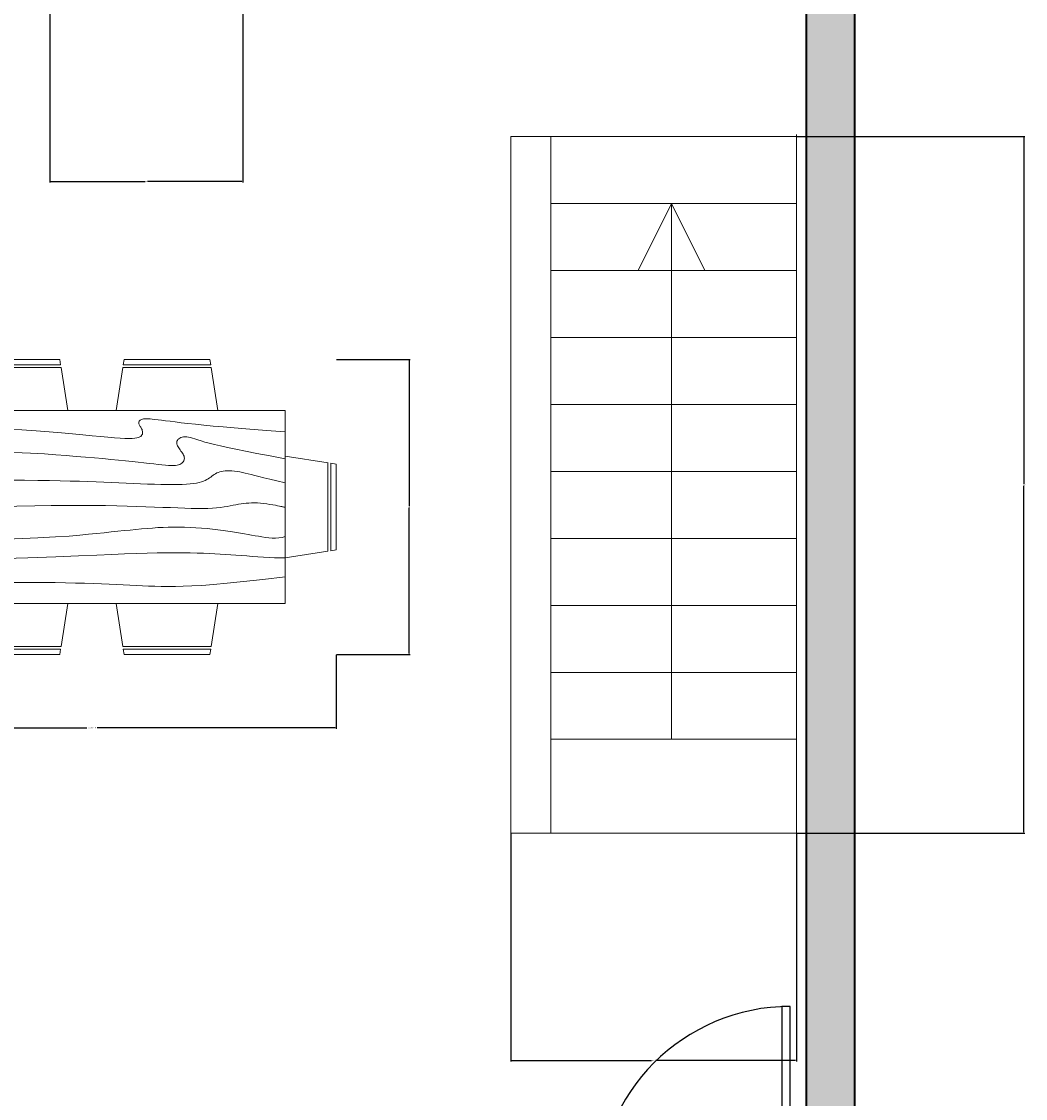
# Model space of a CAD drawing. Units: inches. Extents: x 1563 to 2428, y 777 to 1464.
# Tile 7 of 11: x 1810 to 1997, y 1063 to 1263. Entities that reach past the tile are written whole.
import ezdxf

# ---------------------------------------------------------------- set-up
doc = ezdxf.new("R2010")
doc.units = ezdxf.units.IN
for name, color, linetype, lineweight in [('A-ANNO-DIMS', 2, 'Continuous', 18), ('A-DOOR', 4, 'Continuous', 25), ('A-FLOR-STRS', 7, 'Continuous', 18), ('A-FURN', 9, 'Continuous', 18), ('A-WALL', 7, 'Continuous', 35), ('A-WALL-PATT', 8, 'Continuous', 13)]:
    doc.layers.add(name, color=color, linetype=linetype, lineweight=lineweight)
doc.styles.get("Standard").update_dxf_attribs({"font": 'arial.ttf'})
doc.dimstyles.get("Standard").update_dxf_attribs({"dimtxt": 0.18, "dimasz": 0.18, "dimexe": 0.18, "dimexo": 0.0625, "dimgap": 0.09, "dimtad": 0, "dimtih": 1, "dimtoh": 1, "dimdec": 4, "dimzin": 0, "dimdsep": 46, "dimtxsty": 'Standard', "dimcen": 0.09, "dimadec": 0, "dimazin": 0, "dimtfac": 1, "dimtdec": 4, "dimtofl": 0, "dimtmove": 0, "dimatfit": 3, "dimfxl": 1, "dimtolj": 1, "dimtzin": 0, "dimarcsym": 0})

# ---------------------------------------------------------------- blocks, each defined once
blk = doc.blocks.new('*U3')
for p, q in [((0, 0), (0, -6)), ((-40, 0), (-40, -6))]:
    blk.add_line(p, q)
blk.add_lwpolyline([(0, 0), (0, 40), (-1.75, 40), (-1.75, 0)], close=True)
blk.add_arc((0, 0), 40, 90, 180)
blk = doc.blocks.new('Dining Set - 36 x 72 in.')
for p, q in [((-22, 27.5), (-22.1562, 26.50042)), ((-5.8416, 26.5), (-22.1534, 26.5)), ((-22, 27.5), (-6, 27.5)), ((-5.8437, 26.49966), (-6, 27.5)), ((6, 27.5), (5.8438, 26.50042)), ((22.1584, 26.5), (5.8466, 26.5)), ((6, 27.5), (22, 27.5)), ((22.1563, 26.49966), (22, 27.5)), ((-22.2343, 26.00059), (-23.4847, 17.99762)), ((-22.2304, 26), (-5.7608, 26)), ((-4.5152, 17.99762), (-5.7655, 25.99926)), ((5.7657, 26.00059), (4.5153, 17.99762)), ((5.7696, 26), (22.2392, 26)), ((23.4848, 17.99762), (22.2345, 25.99926)), ((36, 18), (-36, 18)), ((-36, 18), (-36, -18)), ((36, -18), (36, 18)), ((-45.5, 8), (-44.5004, 8.15617)), ((-44.5, -8.15843), (-44.5, 8.15338)), ((-44.0006, 8.23428), (-35.9976, 9.48474)), ((-44, 8.23041), (-44, -8.23915)), ((44.0006, 8.23428), (35.9976, 9.48474)), ((44, 8.23041), (44, -8.23915)), ((44.5, -8.15843), (44.5, 8.15338)), ((45.5, 8), (44.5005, 8.15617)), ((-45.5, 8), (-45.5, -8)), ((45.5, 8), (45.5, -8)), ((-44.4997, -8.15631), (-45.5, -8)), ((44.4997, -8.15631), (45.5, -8)), ((-35.9976, -9.48476), (-43.9993, -8.2345)), ((35.9976, -9.48476), (43.9993, -8.2345)), ((-36, -18), (36, -18)), ((-22.2343, -26.0006), (-23.4847, -17.99762)), ((-4.5152, -17.99762), (-5.7655, -25.99928)), ((5.7657, -26.0006), (4.5153, -17.99762)), ((23.4848, -17.99762), (22.2345, -25.99928)), ((-22.2304, -26), (-5.7608, -26)), ((5.7696, -26), (22.2392, -26)), ((-22, -27.5), (-22.1562, -26.50044)), ((-5.8416, -26.5), (-22.1534, -26.5)), ((-22, -27.5), (-6, -27.5)), ((-5.8437, -26.49967), (-6, -27.5)), ((6, -27.5), (5.8438, -26.50044)), ((22.1584, -26.5), (5.8466, -26.5)), ((6, -27.5), (22, -27.5)), ((22.1563, -26.49967), (22, -27.5))]:
    blk.add_line(p, q)
for points in [[(-36, 15), (-31.1772, 14.97754), (-26.8079, 14.91406), (-22.8538, 14.81543), (-19.276, 14.6875), (-16.0362, 14.53613), (-13.0957, 14.36718), (-10.4159, 14.18652), (-7.9583, 14), (-5.6904, 13.81315), (-3.6035, 13.63021), (-1.6954, 13.45508), (0.0365, 13.29166), (1.5945, 13.14388), (2.9811, 13.01562), (4.1988, 12.9108), (5.25, 12.83333), (6.1393, 12.78613), (6.8802, 12.76823), (7.4883, 12.77767), (7.9792, 12.8125), (8.3685, 12.87077), (8.6719, 12.95052), (8.9049, 13.0498), (9.0833, 13.16666), (9.2205, 13.29899), (9.3216, 13.44401), (9.3895, 13.59879), (9.4271, 13.76041), (9.4373, 13.92594), (9.4232, 14.09245), (9.3875, 14.257), (9.3333, 14.41666), (9.2638, 14.56917), (9.1836, 14.71484), (9.0975, 14.85465), (9.0104, 14.98958), (8.9272, 15.1206), (8.8529, 15.2487), (8.7922, 15.37483), (8.75, 15.5), (8.7305, 15.62467), (8.7344, 15.74739), (8.7617, 15.86621), (8.8125, 15.97916), (8.8867, 16.08431), (8.9844, 16.17968), (9.1055, 16.26334), (9.25, 16.33333), (9.4189, 16.38802), (9.6172, 16.42708), (9.8506, 16.45052), (10.125, 16.45833), (10.4463, 16.45052), (10.8203, 16.42708), (11.2529, 16.38802), (11.75, 16.33333), (12.3184, 16.26318), (12.9694, 16.17838), (13.7151, 16.07991), (14.5677, 15.96875), (15.5395, 15.84586), (16.6426, 15.71224), (17.8893, 15.56884), (19.2917, 15.41666), (20.859, 15.25667), (22.5879, 15.08984), (24.4721, 14.91715), (26.5052, 14.73958), (28.6809, 14.5581), (30.9929, 14.3737), (33.4347, 14.18733), (36, 14)], [(-36, 10), (-28.9766, 10.14274), (-23.1725, 10.20442), (-18.4241, 10.19775), (-14.5677, 10.13541), (-11.4399, 10.03011), (-8.877, 9.89453), (-6.7154, 9.74137), (-4.7917, 9.58333), (-2.9698, 9.43082), (-1.2246, 9.28515), (0.4415, 9.14534), (2.026, 9.01041), (3.5266, 8.87939), (4.9408, 8.7513), (6.266, 8.62516), (7.5, 8.5), (8.6411, 8.37549), (9.6914, 8.2539), (10.6538, 8.13818), (11.5312, 8.03125), (12.3267, 7.93603), (13.043, 7.85547), (13.6831, 7.79248), (14.25, 7.75), (14.7471, 7.7303), (15.1797, 7.73307), (15.5537, 7.75732), (15.875, 7.80208), (16.1494, 7.86637), (16.3828, 7.94922), (16.5811, 8.04964), (16.75, 8.16666), (16.8944, 8.29915), (17.0143, 8.44531), (17.1089, 8.60319), (17.1771, 8.77083), (17.218, 8.94629), (17.2305, 9.1276), (17.2137, 9.31282), (17.1667, 9.5), (17.0895, 9.6875), (16.987, 9.875), (16.8649, 10.0625), (16.7292, 10.25), (16.5856, 10.4375), (16.4401, 10.625), (16.2985, 10.8125), (16.1667, 11), (16.05, 11.18733), (15.9518, 11.3737), (15.8752, 11.5581), (15.8229, 11.73958), (15.798, 11.91715), (15.8034, 12.08984), (15.842, 12.25667), (15.9167, 12.41666), (16.0295, 12.56836), (16.1784, 12.70833), (16.3605, 12.83268), (16.5729, 12.9375), (16.8127, 13.01888), (17.0768, 13.07291), (17.3625, 13.0957), (17.6667, 13.08333), (17.9894, 13.03312), (18.3418, 12.94726), (18.7382, 12.82918), (19.1927, 12.68229), (19.7195, 12.51001), (20.3327, 12.31575), (21.0465, 12.10294), (21.875, 11.875), (22.8357, 11.63354), (23.959, 11.37304), (25.2786, 11.08618), (26.8282, 10.76562), (28.6414, 10.40405), (30.752, 9.99414), (33.1936, 9.52856), (36, 9)], [(-36, 5.5), (-30.7157, 5.3348), (-26.069, 5.20963), (-21.9946, 5.11767), (-18.4271, 5.05208), (-15.3009, 5.00602), (-12.5508, 4.97265), (-10.1112, 4.94515), (-7.9167, 4.91666), (-5.909, 4.88167), (-4.0586, 4.83984), (-2.3429, 4.79215), (-0.7396, 4.73958), (0.7739, 4.6831), (2.22, 4.6237), (3.6213, 4.56233), (5, 4.5), (6.373, 4.43782), (7.7344, 4.3776), (9.0723, 4.32129), (10.375, 4.27083), (11.6309, 4.22819), (12.8281, 4.19531), (13.9551, 4.17415), (15, 4.16666), (15.954, 4.17448), (16.819, 4.19791), (17.6001, 4.23698), (18.3021, 4.29166), (18.9299, 4.36198), (19.4883, 4.44791), (19.9823, 4.54948), (20.4167, 4.66666), (20.7969, 4.79899), (21.1302, 4.94401), (21.4245, 5.09879), (21.6875, 5.26041), (21.9271, 5.42594), (22.1511, 5.59245), (22.3672, 5.757), (22.5834, 5.91666), (22.8065, 6.06868), (23.0404, 6.21093), (23.2879, 6.34147), (23.5521, 6.45833), (23.8358, 6.55957), (24.142, 6.64323), (24.4735, 6.70735), (24.8334, 6.75), (25.2235, 6.76969), (25.642, 6.76692), (26.0858, 6.74267), (26.5521, 6.69791), (27.0379, 6.63362), (27.5404, 6.55078), (28.0565, 6.45036), (28.5834, 6.33333), (29.1242, 6.19987), (29.7071, 6.04687), (30.3661, 5.87044), (31.1354, 5.66666), (32.0493, 5.43164), (33.142, 5.16146), (34.4475, 4.85221), (36, 4.5)], [(-36, -1), (-30.7915, -0.6591), (-26.0195, -0.38216), (-21.6519, -0.16284), (-17.6563, 0.00521), (-14.0005, 0.12833), (-10.6523, 0.21289), (-7.5796, 0.26522), (-4.75, 0.29166), (-2.134, 0.29793), (0.2878, 0.28711), (2.5317, 0.26163), (4.6146, 0.22396), (6.5529, 0.17651), (8.3633, 0.12174), (10.0623, 0.06209), (11.6667, 0), (13.1899, -0.06201), (14.6341, -0.1211), (15.9982, -0.17432), (17.2813, -0.21875), (18.4823, -0.25147), (19.6003, -0.26953), (20.6343, -0.27002), (21.5834, -0.25), (22.4481, -0.20768), (23.2357, -0.14584), (23.9549, -0.06836), (24.6146, 0.02083), (25.2235, 0.11784), (25.7904, 0.21875), (26.3241, 0.31966), (26.8334, 0.41666), (27.3265, 0.50618), (27.8099, 0.58593), (28.2894, 0.65397), (28.7709, 0.70833), (29.2601, 0.74707), (29.763, 0.76823), (30.2855, 0.76985), (30.8334, 0.75), (31.4088, 0.70784), (31.9994, 0.64713), (32.589, 0.57275), (33.1615, 0.48958), (33.7008, 0.4025), (34.1908, 0.3164), (34.6153, 0.23616), (34.9584, 0.16666), (35.2099, 0.11165), (35.3848, 0.07031), (35.504, 0.04069), (35.5886, 0.02083), (35.6594, 0.00879), (35.7377, 0.0026), (35.8442, 0.00032), (36, 0)], [(-36, -6.5), (-27.1843, -6.31267), (-20.084, -6.1263), (-14.469, -5.9419), (-10.1094, -5.76042), (-6.7752, -5.58285), (-4.2363, -5.41016), (-2.2629, -5.24333), (-0.625, -5.08334), (0.8708, -4.93099), (2.2715, -4.78646), (3.5872, -4.64974), (4.8281, -4.52084), (6.0046, -4.39974), (7.127, -4.28646), (8.2053, -4.18099), (9.25, -4.08334), (10.2705, -3.99382), (11.2734, -3.91407), (12.2647, -3.84603), (13.25, -3.79167), (14.2354, -3.75293), (15.2266, -3.73177), (16.2295, -3.73015), (17.25, -3.75), (18.2912, -3.79248), (19.3451, -3.85547), (20.4009, -3.93604), (21.4479, -4.03125), (22.4754, -4.13819), (23.4727, -4.25391), (24.4289, -4.37549), (25.3334, -4.5), (26.1785, -4.62492), (26.9694, -4.74935), (27.7145, -4.87281), (28.4219, -4.99479), (29.1, -5.11483), (29.7572, -5.23242), (30.4016, -5.34709), (31.0417, -5.45834), (31.6837, -5.56437), (32.3262, -5.65821), (32.9658, -5.73153), (33.599, -5.77604), (34.2224, -5.78345), (34.8327, -5.74545), (35.4264, -5.65373), (36, -5.5)], [(-36, -10), (-26.4022, -9.81299), (-18.4675, -9.62891), (-11.9839, -9.45069), (-6.7396, -9.28125), (-2.5226, -9.12354), (0.8789, -8.98047), (3.6769, -8.85498), (6.0833, -8.75), (8.2767, -8.66765), (10.3021, -8.60677), (12.1712, -8.56543), (13.8958, -8.54167), (15.4876, -8.53353), (16.9583, -8.53907), (18.3197, -8.55632), (19.5834, -8.58334), (20.7616, -8.61841), (21.8685, -8.66081), (22.9188, -8.71004), (23.9271, -8.76563), (24.9081, -8.82707), (25.8763, -8.89388), (26.8465, -8.96558), (27.8334, -9.04167), (28.8474, -9.12118), (29.8828, -9.20117), (30.93, -9.27824), (31.9792, -9.34896), (33.0205, -9.40991), (34.0443, -9.45768), (35.0407, -9.48885), (36, -9.5)], [(-36, -14.5), (-30.0881, -14.33513), (-25.0332, -14.21224), (-20.7312, -14.12647), (-17.0781, -14.07292), (-13.97, -14.04671), (-11.3027, -14.04297), (-8.9724, -14.05681), (-6.875, -14.08334), (-4.9224, -14.11833), (-3.0905, -14.16016), (-1.3709, -14.20785), (0.2448, -14.26042), (1.7647, -14.3169), (3.1973, -14.3763), (4.5507, -14.43767), (5.8333, -14.5), (7.0554, -14.5621), (8.235, -14.62175), (9.3922, -14.67652), (10.5469, -14.72396), (11.7192, -14.76164), (12.929, -14.78711), (14.1965, -14.79794), (15.5417, -14.79167), (16.9933, -14.76424), (18.6152, -14.70508), (20.4804, -14.60197), (22.6615, -14.44271), (25.2312, -14.21509), (28.2624, -13.9069), (31.8277, -13.50594), (36, -13)]]:
    blk.add_lwpolyline(points)
blk = doc.blocks.new('*D42')
at = {"layer": 'A-ANNO-DIMS', "color": 0, "lineweight": -2, "transparency": 16777216}
for p, q in [((1777.49, 1145.29), (1777.49, 1131.52)), ((1868.49, 1145.29), (1868.49, 1131.52)), ((1777.67, 1131.7), (1822.03, 1131.7)), ((1868.31, 1131.7), (1823.94, 1131.7))]:
    blk.add_line(p, q, dxfattribs=at)
at = {"layer": 'A-ANNO-DIMS', "color": 0, "transparency": 16777216}
for points in [[(1777.67, 1131.73), (1777.67, 1131.67), (1777.49, 1131.7)], [(1868.31, 1131.73), (1868.31, 1131.67), (1868.49, 1131.7)]]:
    blk.add_solid(points, dxfattribs=at)
at = {"layer": 'Defpoints', "color": 0, "transparency": 16777216}
for p in [(1777.49, 1145.35), (1868.49, 1145.35), (1868.49, 1131.7)]:
    blk.add_point(p, dxfattribs=at)
at = {"layer": 'A-ANNO-DIMS', "color": 0, "transparency": 16777216, "insert": (1822.99, 1131.7), "char_height": 0.18, "attachment_point": 5}
blk.add_mtext('\\A1;DINING SET 91', dxfattribs=at)
blk = doc.blocks.new('*D43')
at = {"layer": 'A-ANNO-DIMS', "color": 0, "lineweight": -2, "transparency": 16777216}
for p, q in [((1868.55, 1200.35), (1882.32, 1200.35)), ((1882.14, 1200.17), (1882.14, 1173.03)), ((1882.14, 1145.53), (1882.14, 1172.67)), ((1868.55, 1145.35), (1882.32, 1145.35))]:
    blk.add_line(p, q, dxfattribs=at)
at = {"layer": 'A-ANNO-DIMS', "color": 0, "transparency": 16777216}
for points in [[(1882.11, 1200.17), (1882.17, 1200.17), (1882.14, 1200.35)], [(1882.11, 1145.53), (1882.17, 1145.53), (1882.14, 1145.35)]]:
    blk.add_solid(points, dxfattribs=at)
at = {"layer": 'Defpoints', "color": 0, "transparency": 16777216}
for p in [(1868.49, 1200.35), (1882.14, 1200.35), (1868.49, 1145.35)]:
    blk.add_point(p, dxfattribs=at)
at = {"layer": 'A-ANNO-DIMS', "color": 0, "transparency": 16777216, "insert": (1882.14, 1172.85), "char_height": 0.18, "attachment_point": 5}
blk.add_mtext('\\A1;55', dxfattribs=at)
blk = doc.blocks.new('*D64')
at = {"layer": 'A-ANNO-DIMS', "color": 0, "lineweight": -2, "transparency": 16777216}
for p, q in [((1815.11, 1275.87), (1815.11, 1233.35)), ((1851.11, 1275.87), (1851.11, 1233.35)), ((1815.29, 1233.53), (1832.89, 1233.53)), ((1850.93, 1233.53), (1833.32, 1233.53))]:
    blk.add_line(p, q, dxfattribs=at)
at = {"layer": 'A-ANNO-DIMS', "color": 0, "transparency": 16777216}
for points in [[(1815.29, 1233.56), (1815.29, 1233.5), (1815.11, 1233.53)], [(1850.93, 1233.56), (1850.93, 1233.5), (1851.11, 1233.53)]]:
    blk.add_solid(points, dxfattribs=at)
at = {"layer": 'Defpoints', "color": 0, "transparency": 16777216}
for p in [(1815.11, 1275.93), (1851.11, 1275.93), (1815.11, 1233.53)]:
    blk.add_point(p, dxfattribs=at)
at = {"layer": 'A-ANNO-DIMS', "color": 0, "transparency": 16777216, "insert": (1833.11, 1233.53), "char_height": 0.18, "attachment_point": 5}
blk.add_mtext('\\A1;36', dxfattribs=at)
blk = doc.blocks.new('*D67')
at = {"layer": 'A-ANNO-DIMS', "color": 0, "lineweight": -2, "transparency": 16777216}
for p, q in [((1901.06, 1112.03), (1901.06, 1069.51)), ((1954.3, 1112.03), (1954.3, 1069.51)), ((1901.24, 1069.69), (1927.28, 1069.69)), ((1954.12, 1069.69), (1928.07, 1069.69))]:
    blk.add_line(p, q, dxfattribs=at)
at = {"layer": 'A-ANNO-DIMS', "color": 0, "transparency": 16777216}
for points in [[(1901.24, 1069.72), (1901.24, 1069.66), (1901.06, 1069.69)], [(1954.12, 1069.72), (1954.12, 1069.66), (1954.3, 1069.69)]]:
    blk.add_solid(points, dxfattribs=at)
at = {"layer": 'Defpoints', "color": 0, "transparency": 16777216}
for p in [(1901.06, 1112.09), (1954.3, 1112.09), (1901.06, 1069.69)]:
    blk.add_point(p, dxfattribs=at)
at = {"layer": 'A-ANNO-DIMS', "color": 0, "transparency": 16777216, "insert": (1927.68, 1069.69), "char_height": 0.18, "attachment_point": 5}
blk.add_mtext('\\A1;53.24', dxfattribs=at)
blk = doc.blocks.new('*D68')
at = {"layer": 'A-ANNO-DIMS', "color": 0, "lineweight": -2, "transparency": 16777216}
for p, q in [((1954.36, 1241.89), (1996.88, 1241.89)), ((1996.7, 1241.71), (1996.7, 1177.17)), ((1996.7, 1112.27), (1996.7, 1176.81)), ((1954.36, 1112.09), (1996.88, 1112.09))]:
    blk.add_line(p, q, dxfattribs=at)
at = {"layer": 'A-ANNO-DIMS', "color": 0, "transparency": 16777216}
for points in [[(1996.67, 1241.71), (1996.73, 1241.71), (1996.7, 1241.89)], [(1996.67, 1112.27), (1996.73, 1112.27), (1996.7, 1112.09)]]:
    blk.add_solid(points, dxfattribs=at)
at = {"layer": 'Defpoints', "color": 0, "transparency": 16777216}
for p in [(1954.3, 1241.89), (1954.3, 1112.09), (1996.7, 1112.09)]:
    blk.add_point(p, dxfattribs=at)
at = {"layer": 'A-ANNO-DIMS', "color": 0, "transparency": 16777216, "insert": (1996.7, 1176.99), "char_height": 0.18, "attachment_point": 5}
blk.add_mtext('\\A1;129.8', dxfattribs=at)

msp = doc.modelspace()

# ---------------------------------------------------------------- hatches: boundary and pattern name
at = {"layer": 'A-WALL-PATT'}
h = msp.add_hatch(color=256, dxfattribs=at)
h.dxf.hatch_style = 1
h.paths.add_polyline_path([(1965.105, 1421.428), (1605.105, 1421.428), (1605.105, 821.428), (1965.105, 821.428)])
h.paths.add_polyline_path([(1614.105, 1199.428), (1704.105, 1199.428), (1738.605, 1199.428), (1738.605, 1251.928), (1734.105, 1251.928), (1734.105, 1203.928), (1704.105, 1203.928), (1614.105, 1203.928), (1614.105, 1335.928), (1665.105, 1335.928), (1665.105, 1340.428), (1614.105, 1340.428), (1614.105, 1412.428), (1704.105, 1412.428), (1704.105, 1340.428), (1701.105, 1340.428), (1701.105, 1335.928), (1704.105, 1335.928), (1768.605, 1335.928), (1768.605, 1340.428), (1708.605, 1340.428), (1708.605, 1412.428), (1807.605, 1412.428), (1807.605, 1340.428), (1804.605, 1340.428), (1804.605, 1335.928), (1807.605, 1335.928), (1807.605, 1275.928), (1815.105, 1275.928), (1815.105, 1280.428), (1812.105, 1280.428), (1812.105, 1412.428), (1956.105, 1412.428), (1956.105, 1280.428), (1854.105, 1280.428), (1854.105, 1275.928), (1956.105, 1275.928), (1956.105, 830.428), (1614.105, 830.428)], flags=16)
h.paths.add_polyline_path([(1917.224, 1038.928), (1917.224, 1043.846, -0.4014527), (1951.591, 1079.751), (1951.591, 1079.786), (1953.163, 1079.786), (1953.163, 1043.846), (1953.163, 1038.455), (1953.105, 1034.428), (1953.105, 1038.928), (1953.163, 1043.846), (1951.591, 1043.846), (1951.591, 1079.751, 0.4014527), (1917.224, 1043.846), (1917.224, 1038.455), (1917.224, 1034.428), (1834.605, 1034.428), (1834.605, 906.928), (1858.605, 906.928), (1858.605, 954.928), (1932.105, 954.928), (1932.105, 902.428), (1834.605, 902.428), (1834.605, 1034.428), (1914.224, 1034.428), (1914.224, 1038.928)], flags=0)
edge = h.paths.add_edge_path(flags=0)
edge.add_ellipse((1674.345, 1004.483), major_axis=(1.48, 0), ratio=0.8423039, start_angle=90, end_angle=180, ccw=False)
edge.add_line((1674.345, 1005.73), (1674.921, 1005.73))
edge.add_ellipse((2202.617, 985.642), major_axis=(528.234, 0), ratio=0.8423039, start_angle=176.34957, end_angle=177.82005, ccw=False)
edge.add_ellipse((1739.278, 760.804), major_axis=(-313.308, 0), ratio=0.8423039, start_angle=-77.87403, end_angle=-76.21947, ccw=False)
edge.add_ellipse((1739.278, 767.659), major_axis=(305.303, 0), ratio=0.8423039, start_angle=100.20954, end_angle=102.44463, ccw=False)
edge.add_ellipse((1659.357, 1231.328), major_axis=(250.96, 0), ratio=0.8423039, start_angle=-80.74343, end_angle=-77.44507)
edge.add_line((1705.625, 1023.567), (1711.685, 1026.918))
edge.add_ellipse((1711.754, 1026.21), major_axis=(0.74, 0), ratio=0.8423039, start_angle=52.06687, end_angle=90, ccw=False)
edge.add_line((1712.16, 1026.731), (1717.882, 1023.567))
edge.add_ellipse((1764.151, 1231.328), major_axis=(250.96, 0), ratio=0.8423039, start_angle=257.44507, end_angle=260.74343)
edge.add_ellipse((1684.229, 767.659), major_axis=(305.303, 0), ratio=0.8423039, start_angle=77.55537, end_angle=79.79046, ccw=False)
edge.add_ellipse((1684.229, 760.804), major_axis=(-313.308, 0), ratio=0.8423039, start_angle=256.21947, end_angle=257.87403, ccw=False)
edge.add_ellipse((1220.891, 985.642), major_axis=(-528.234, 0), ratio=0.8423039, start_angle=182.17995, end_angle=183.65043, ccw=False)
edge.add_line((1748.586, 1005.73), (1749.162, 1005.73))
edge.add_ellipse((1749.162, 1004.483), major_axis=(-1.48, 0), ratio=0.8423039, start_angle=180, end_angle=270, ccw=False)
edge.add_line((1750.642, 1004.483), (1750.642, 980.28))
edge.add_ellipse((1749.162, 980.28), major_axis=(1.48, 0), ratio=0.8423039, start_angle=270, end_angle=360, ccw=False)
edge.add_ellipse((-8843.864, 962.352), major_axis=(10593.026, 0), ratio=0.84230387, start_angle=-0.3241203, end_angle=0.0902291, ccw=False)
edge.add_ellipse((-8843.864, 962.352), major_axis=(10593.026, 0), ratio=0.84230387, start_angle=-0.3838668, end_angle=-0.3241203, ccw=False)
edge.add_ellipse((1749.162, 890.136), major_axis=(1.48, 0), ratio=0.8423039, start_angle=0, end_angle=90, ccw=False)
edge.add_line((1750.642, 890.136), (1750.642, 865.933))
edge.add_ellipse((1749.162, 865.933), major_axis=(1.48, 0), ratio=0.8423039, start_angle=270, end_angle=360, ccw=False)
edge.add_line((1749.162, 864.686), (1748.528, 864.686))
edge.add_ellipse((-8843.864, 962.352), major_axis=(10593.026, 0), ratio=0.84230387, start_angle=-0.6186432, end_angle=-0.5282715, ccw=False)
edge.add_ellipse((1747.592, 846.206), major_axis=(-2.22, 0), ratio=0.8423039, start_angle=179.37176, end_angle=248.46476, ccw=False)
edge.add_ellipse((-8844.604, 962.352), major_axis=(-10595.313, 0), ratio=0.842303864, start_angle=179.3534459, end_angle=179.3717628, ccw=False)
edge.add_ellipse((1744.512, 842.854), major_axis=(-5.246, 0), ratio=0.8423039, start_angle=90, end_angle=179.35345, ccw=False)
edge.add_line((1744.512, 838.435), (1678.995, 838.435))
edge.add_ellipse((1678.995, 842.854), major_axis=(5.246, 0), ratio=0.8423039, start_angle=180.64655, end_angle=270, ccw=False)
edge.add_ellipse((12268.111, 962.352), major_axis=(-10595.313, 0), ratio=0.84230387, start_angle=0.6282372, end_angle=0.6465541, ccw=False)
edge.add_ellipse((1675.916, 846.206), major_axis=(-2.22, 0), ratio=0.8423039, start_angle=-68.46476, end_angle=0.62824, ccw=False)
edge.add_ellipse((12267.371, 962.352), major_axis=(-10593.026, 0), ratio=0.84230387, start_angle=0.5282715, end_angle=0.6465541, ccw=False)
edge.add_line((1674.98, 864.686), (1674.345, 864.686))
edge.add_ellipse((1674.345, 865.933), major_axis=(-1.48, 0), ratio=0.8423039, start_angle=0, end_angle=90, ccw=False)
edge.add_line((1672.865, 865.933), (1672.865, 890.136))
edge.add_ellipse((1674.345, 890.136), major_axis=(1.48, 0), ratio=0.8423039, start_angle=90, end_angle=180, ccw=False)
edge.add_ellipse((12267.371, 962.352), major_axis=(-10593.026, 0), ratio=0.84230387, start_angle=0.3241203, end_angle=0.3838668, ccw=False)
edge.add_ellipse((12267.371, 962.352), major_axis=(-10593.026, 0), ratio=0.84230387, start_angle=-0.0902291, end_angle=0.3241203, ccw=False)
edge.add_ellipse((1674.345, 980.28), major_axis=(-1.48, 0), ratio=0.8423039, start_angle=0, end_angle=90, ccw=False)
edge.add_line((1672.865, 980.28), (1672.865, 1004.483))
h.paths.add_polyline_path([(1622.542, 1135.584), (1648.534, 1136.233), (1648.683, 1130.234), (1647.126, 1130.196), (1648.323, 1082.21), (1649.88, 1082.249), (1650.03, 1076.251), (1624.038, 1075.603, -0.266667)], flags=0)
edge = h.paths.add_edge_path(flags=0)
edge.add_line((1694.584, 990.705), (1700.334, 994.711))
edge.add_line((1700.334, 994.711), (1702.248, 994.711))
edge.add_line((1702.248, 994.711), (1702.248, 997.061))
edge.add_ellipse((1758.417, 997.061), major_axis=(56.169, 0), ratio=0.8423039, start_angle=150.56143, end_angle=180, ccw=False)
edge.add_ellipse((1665.091, 997.061), major_axis=(-56.169, 0), ratio=0.8423039, start_angle=180, end_angle=209.43857, ccw=False)
edge.add_line((1721.26, 997.061), (1721.26, 994.711))
edge.add_line((1721.26, 994.711), (1723.174, 994.711))
edge.add_line((1723.174, 994.711), (1728.923, 990.705))
edge.add_line((1728.923, 990.705), (1728.923, 975.895))
edge.add_ellipse((1725.091, 976.043), major_axis=(0.357, 6.34), ratio=0.6038336, start_angle=106.34259, end_angle=270.99799, ccw=False)
edge.add_line((1721.26, 975.15), (1721.26, 997.061))
edge.add_ellipse((1665.091, 997.061), major_axis=(-56.169, 0), ratio=0.8423039, start_angle=180, end_angle=209.43857)
edge.add_ellipse((1758.417, 997.061), major_axis=(56.169, 0), ratio=0.8423039, start_angle=150.56143, end_angle=180)
edge.add_line((1702.248, 997.061), (1702.248, 975.15))
edge.add_ellipse((1698.416, 976.043), major_axis=(-0.357, 6.34), ratio=0.6038336, start_angle=89.00201, end_angle=253.65741, ccw=False)
edge.add_line((1694.584, 975.895), (1694.584, 990.705))
edge = h.paths.add_edge_path(flags=0)
edge.add_line((1675.832, 952.075), (1679.883, 938.848))
edge.add_ellipse((5378.107, 931.045), major_axis=(-3698.236, 0), ratio=0.84230387, start_angle=-0.120897, end_angle=0.364076)
edge.add_line((1679.976, 907.545), (1676.149, 892.52))
edge.add_ellipse((12267.371, 962.352), major_axis=(10591.546, 0), ratio=0.84230387, start_angle=180.3241656, end_angle=180.3777642, ccw=False)
edge.add_ellipse((12267.371, 962.352), major_axis=(10591.546, 0), ratio=0.84230387, start_angle=180.0555943, end_angle=180.3241656, ccw=False)
edge = h.paths.add_edge_path(flags=0)
edge.add_ellipse((1706.366, 891.542), major_axis=(81.773, 0), ratio=0.8423039, start_angle=94.27742, end_angle=111.83495, ccw=False)
edge.add_line((1701.225, 960.283), (1722.283, 960.283))
edge.add_ellipse((1717.141, 891.542), major_axis=(-81.773, 0), ratio=0.8423039, start_angle=248.16505, end_angle=265.72258, ccw=False)
edge.add_line((1743.29, 956.803), (1741.105, 940.427))
edge.add_ellipse((1714.553, 877.238), major_axis=(79.58, 0), ratio=0.8423039, start_angle=67.20809, end_angle=85.12993)
edge.add_line((1720.25, 944.097), (1703.258, 944.097))
edge.add_ellipse((1708.954, 877.238), major_axis=(79.58, 0), ratio=0.8423039, start_angle=94.87007, end_angle=112.79191)
edge.add_line((1682.403, 940.427), (1680.218, 956.803))
h.paths.add_polyline_path([(1664.992, 1093.991), (1664.992, 1123.991), (1724.992, 1123.991), (1724.992, 1093.991)], flags=0)
h.paths.add_polyline_path([(1716.588, 1099.729), (1715.404, 1099.805), (1715.021, 1099.823), (1716.177, 1099.758)], flags=0)
h.paths.add_polyline_path([(1711.325, 1103.757), (1712.167, 1103.706), (1713.009, 1103.642), (1713.84, 1103.566), (1715.041, 1103.439), (1716.532, 1103.244), (1717.793, 1103.048), (1718.876, 1102.854), (1719.676, 1102.699), (1720.157, 1102.605), (1720.632, 1102.513), (1721.109, 1102.424), (1721.595, 1102.339), (1722.088, 1102.264), (1722.585, 1102.205), (1723.082, 1102.17), (1723.575, 1102.164), (1724.321, 1102.211), (1724.533, 1102.268), (1723.842, 1102.16), (1722.864, 1102.172), (1721.894, 1102.287), (1720.935, 1102.454), (1720.157, 1102.605), (1719.676, 1102.699), (1719.18, 1102.795), (1718.66, 1102.892), (1718.109, 1102.991), (1717.517, 1103.091), (1716.876, 1103.191), (1716.179, 1103.29), (1715.435, 1103.387), (1714.652, 1103.48), (1713.84, 1103.566), (1713.009, 1103.642), (1712.167, 1103.706), (1711.325, 1103.757), (1710.492, 1103.791), (1709.676, 1103.806), (1708.873, 1103.805), (1707.707, 1103.78), (1707.292, 1103.757), (1708.499, 1103.805), (1710.086, 1103.807)], flags=0)
h.paths.add_polyline_path([(1713.959, 1106.591), (1714.651, 1106.624), (1715.279, 1106.674), (1715.852, 1106.736), (1716.373, 1106.807), (1716.851, 1106.885), (1717.289, 1106.966), (1717.696, 1107.046), (1718.341, 1107.178), (1719.173, 1107.331), (1720.169, 1107.421), (1721.131, 1107.383), (1722.032, 1107.286), (1722.934, 1107.152), (1723.887, 1106.983), (1724.746, 1106.795), (1724.72, 1106.798), (1724.663, 1106.807), (1724.241, 1106.906), (1724.159, 1106.924), (1723.885, 1106.979), (1723.546, 1107.044), (1723.157, 1107.113), (1722.732, 1107.182), (1722.284, 1107.249), (1721.827, 1107.308), (1721.375, 1107.357), (1720.942, 1107.391), (1720.539, 1107.406), (1720.162, 1107.405), (1719.804, 1107.388), (1719.459, 1107.357), (1719.12, 1107.314), (1718.781, 1107.259), (1718.435, 1107.195), (1718.076, 1107.124), (1717.402, 1106.986), (1716.59, 1106.837), (1715.56, 1106.696), (1714.317, 1106.598)], flags=0)
h.paths.add_polyline_path([(1708.692, 1110.124), (1709.455, 1110.13), (1710.147, 1110.149), (1710.772, 1110.18), (1711.334, 1110.224), (1711.836, 1110.28), (1712.283, 1110.349), (1712.678, 1110.43), (1713.026, 1110.524), (1713.33, 1110.63), (1713.596, 1110.746), (1713.832, 1110.87), (1714.042, 1110.999), (1714.234, 1111.131), (1714.413, 1111.264), (1714.586, 1111.396), (1715.065, 1111.75), (1715.879, 1112.11), (1716.842, 1112.224), (1717.903, 1112.165), (1719.048, 1111.965), (1719.867, 1111.736), (1720.686, 1111.487), (1721.596, 1111.22), (1721.917, 1111.136), (1721.028, 1111.383), (1720.222, 1111.628), (1719.815, 1111.75), (1719.434, 1111.857), (1719.054, 1111.951), (1718.672, 1112.031), (1718.292, 1112.097), (1717.918, 1112.149), (1717.554, 1112.185), (1717.204, 1112.204), (1716.871, 1112.206), (1716.559, 1112.191), (1716.271, 1112.156), (1716.006, 1112.105), (1715.761, 1112.038), (1715.534, 1111.957), (1715.323, 1111.864), (1715.125, 1111.759), (1714.937, 1111.645), (1714.759, 1111.524), (1714.586, 1111.396), (1714.413, 1111.264), (1714.003, 1110.96), (1713.331, 1110.606), (1712.501, 1110.382), (1711.61, 1110.245), (1710.489, 1110.158), (1709.111, 1110.121)], flags=0)
h.paths.add_polyline_path([(1707.127, 1113.075), (1707.639, 1113.025), (1708.092, 1112.991), (1708.49, 1112.975), (1708.836, 1112.977), (1709.135, 1112.996), (1709.392, 1113.032), (1709.612, 1113.084), (1709.798, 1113.15), (1709.957, 1113.23), (1710.092, 1113.324), (1710.208, 1113.431), (1710.304, 1113.554), (1710.379, 1113.698), (1710.434, 1113.866), (1710.467, 1114.062), (1710.477, 1114.289), (1710.463, 1114.553), (1710.426, 1114.857), (1710.364, 1115.202), (1710.282, 1115.58), (1710.184, 1115.98), (1710.076, 1116.391), (1709.961, 1116.801), (1709.844, 1117.201), (1709.731, 1117.579), (1709.626, 1117.924), (1709.532, 1118.228), (1709.454, 1118.493), (1709.392, 1118.723), (1709.351, 1118.924), (1709.293, 1119.435), (1709.831, 1119.942), (1710.705, 1120.121), (1711.507, 1119.898), (1712.224, 1119.567), (1713.189, 1119.016), (1713.529, 1118.804), (1712.958, 1119.148), (1712.468, 1119.428), (1712.046, 1119.649), (1711.683, 1119.817), (1711.366, 1119.937), (1711.084, 1120.016), (1710.826, 1120.057), (1710.582, 1120.067), (1710.354, 1120.049), (1710.142, 1120.006), (1709.951, 1119.941), (1709.781, 1119.857), (1709.635, 1119.757), (1709.516, 1119.645), (1709.426, 1119.524), (1709.366, 1119.395), (1709.335, 1119.255), (1709.331, 1119.1), (1709.351, 1118.924), (1709.392, 1118.723), (1709.454, 1118.493), (1709.52, 1118.268), (1709.799, 1117.356), (1710.028, 1116.57), (1710.245, 1115.749), (1710.45, 1114.804), (1710.477, 1114.289), (1710.448, 1113.654), (1709.908, 1113.153), (1709.165, 1112.979), (1708.318, 1112.974), (1707.448, 1113.039)], flags=0)
h.paths.add_polyline_path([(1700.892, 1119.857), (1701.604, 1119.819), (1702.196, 1119.805), (1702.683, 1119.813), (1703.076, 1119.841), (1703.387, 1119.887), (1703.63, 1119.951), (1703.816, 1120.03), (1703.959, 1120.124), (1704.069, 1120.23), (1704.15, 1120.346), (1704.204, 1120.47), (1704.234, 1120.599), (1704.242, 1120.731), (1704.231, 1120.864), (1704.202, 1120.996), (1704.159, 1121.124), (1704.103, 1121.246), (1704.039, 1121.362), (1703.97, 1121.474), (1703.901, 1121.582), (1703.834, 1121.687), (1703.775, 1121.79), (1703.564, 1122.226), (1704.048, 1122.698), (1704.756, 1122.769), (1705.49, 1122.723), (1706.24, 1122.641), (1706.547, 1122.601), (1706.092, 1122.657), (1705.695, 1122.701), (1705.348, 1122.732), (1705.049, 1122.751), (1704.792, 1122.757), (1704.573, 1122.751), (1704.386, 1122.732), (1704.227, 1122.701), (1704.092, 1122.657), (1703.977, 1122.601), (1703.88, 1122.534), (1703.802, 1122.458), (1703.742, 1122.374), (1703.702, 1122.284), (1703.68, 1122.188), (1703.677, 1122.09), (1703.692, 1121.991), (1703.726, 1121.89), (1703.769, 1121.802), (1704.039, 1121.362), (1704.301, 1120.887), (1704.133, 1120.165), (1703.43, 1119.866), (1702.481, 1119.798), (1701.306, 1119.827)], flags=0)
edge = h.paths.add_edge_path(flags=0)
edge.add_ellipse((1711.754, 1009.752), major_axis=(-147.018, 0), ratio=0.8423039, start_angle=76.40187, end_angle=103.59813)
edge.add_line((1741.105, 888.411), (1741.105, 869.587))
edge.add_ellipse((1711.754, 990.928), major_axis=(-147.018, 0), ratio=0.8423039, start_angle=76.40187, end_angle=103.59813, ccw=False)
edge.add_line((1682.403, 869.587), (1682.403, 888.411))
edge = h.paths.add_edge_path(flags=0)
edge.add_ellipse((-8843.864, 962.352), major_axis=(-10591.546, 0), ratio=0.84230387, start_angle=179.6758344, end_angle=179.9444057, ccw=False)
edge.add_ellipse((-8843.864, 962.352), major_axis=(-10591.546, 0), ratio=0.84230387, start_angle=179.6222358, end_angle=179.6758344, ccw=False)
edge.add_line((1747.358, 892.52), (1743.531, 907.545))
edge.add_ellipse((-1954.6, 931.045), major_axis=(3698.236, 0), ratio=0.84230387, start_angle=-0.364076, end_angle=0.120897)
edge.add_line((1743.625, 938.848), (1747.676, 952.075))
h.paths.add_polyline_path([(1637.931, 1162.087), (1637.931, 1188.087, -0.1904762), (1721.931, 1188.087), (1721.931, 1162.087), (1715.931, 1162.087), (1715.931, 1163.644), (1643.931, 1163.644), (1643.931, 1162.087)], flags=0)
h.paths.add_polyline_path([(1667.931, 1189.491, -0.0496282), (1691.931, 1189.491), (1691.931, 1182.705), (1667.931, 1182.705)], flags=0)
edge = h.paths.add_edge_path(flags=0)
edge.add_ellipse((1685.362, 859.825), major_axis=(-2.96, 0), ratio=0.8423039, start_angle=-90, end_angle=0, ccw=False)
edge.add_line((1685.362, 862.318), (1738.145, 862.318))
edge.add_ellipse((1738.145, 859.825), major_axis=(2.96, 0), ratio=0.8423039, start_angle=0, end_angle=90, ccw=False)
edge.add_line((1741.105, 859.825), (1741.105, 840.361))
edge.add_line((1741.105, 840.361), (1682.403, 840.361))
edge.add_line((1682.403, 840.361), (1682.403, 859.825))
h.paths.add_polyline_path([(1777.486, 1164.853), (1777.486, 1180.853), (1778.486, 1181.01), (1778.486, 1164.697)], flags=0)
h.paths.add_polyline_path([(1786.986, 1154.853), (1786.986, 1163.369), (1778.986, 1164.619), (1778.986, 1181.088), (1786.986, 1182.338), (1786.986, 1190.853), (1799.502, 1190.853), (1800.752, 1198.853), (1817.221, 1198.853), (1818.471, 1190.853), (1827.502, 1190.853), (1828.752, 1198.853), (1845.221, 1198.853), (1846.471, 1190.853), (1858.986, 1190.853), (1858.986, 1182.338), (1866.986, 1181.088), (1866.986, 1164.619), (1858.986, 1163.369), (1858.986, 1154.853), (1846.471, 1154.853), (1845.221, 1146.853), (1828.752, 1146.853), (1827.502, 1154.853), (1818.471, 1154.853), (1817.221, 1146.853), (1800.752, 1146.853), (1799.502, 1154.853)], flags=0)
h.paths.add_polyline_path([(1800.986, 1145.353), (1800.83, 1146.353), (1817.143, 1146.353), (1816.986, 1145.353)], flags=0)
h.paths.add_polyline_path([(1851.408, 1167.858), (1852.086, 1167.738), (1852.744, 1167.621), (1853.388, 1167.506), (1854.028, 1167.395), (1854.67, 1167.289), (1855.313, 1167.195), (1855.952, 1167.122), (1856.585, 1167.077), (1857.209, 1167.07), (1858.147, 1167.128), (1858.413, 1167.2), (1857.547, 1167.066), (1856.312, 1167.08), (1855.07, 1167.223), (1854.028, 1167.395), (1853.388, 1167.506), (1852.744, 1167.621), (1852.086, 1167.738), (1851.408, 1167.858), (1850.288, 1168.052), (1849.956, 1168.104), (1850.701, 1167.98)], flags=0)
h.paths.add_polyline_path([(1845.435, 1172.646), (1846.222, 1172.707), (1846.941, 1172.785), (1847.601, 1172.874), (1848.21, 1172.971), (1848.777, 1173.072), (1849.311, 1173.173), (1850.14, 1173.331), (1851.063, 1173.483), (1852.014, 1173.591), (1853.012, 1173.633), (1854.075, 1173.594), (1855.251, 1173.473), (1856.4, 1173.306), (1857.391, 1173.132), (1857.945, 1173.02), (1858.196, 1172.965), (1858.595, 1172.871), (1858.575, 1172.874), (1858.49, 1172.894), (1858.371, 1172.924), (1858.196, 1172.965), (1857.945, 1173.02), (1857.602, 1173.089), (1857.177, 1173.17), (1856.687, 1173.256), (1856.148, 1173.343), (1855.575, 1173.426), (1854.986, 1173.5), (1854.395, 1173.561), (1853.82, 1173.603), (1853.272, 1173.623), (1852.749, 1173.622), (1852.247, 1173.6), (1851.757, 1173.562), (1851.276, 1173.507), (1850.796, 1173.439), (1850.313, 1173.359), (1849.82, 1173.27), (1849.311, 1173.173), (1848.421, 1173.005), (1847.25, 1172.818), (1845.826, 1172.665)], flags=0)
h.paths.add_polyline_path([(1840.587, 1177.09), (1841.289, 1177.145), (1841.916, 1177.215), (1842.475, 1177.301), (1842.969, 1177.403), (1843.403, 1177.52), (1843.783, 1177.652), (1844.117, 1177.797), (1844.411, 1177.952), (1844.674, 1178.114), (1844.914, 1178.279), (1845.138, 1178.446), (1845.644, 1178.831), (1846.285, 1179.221), (1847.125, 1179.521), (1847.998, 1179.624), (1848.834, 1179.619), (1849.768, 1179.529), (1850.775, 1179.363), (1851.78, 1179.14), (1852.111, 1179.053), (1851.57, 1179.187), (1851.043, 1179.304), (1850.527, 1179.404), (1850.024, 1179.487), (1849.539, 1179.551), (1849.072, 1179.596), (1848.628, 1179.62), (1848.21, 1179.623), (1847.82, 1179.603), (1847.46, 1179.561), (1847.128, 1179.497), (1846.822, 1179.413), (1846.539, 1179.312), (1846.274, 1179.195), (1846.027, 1179.064), (1845.793, 1178.922), (1845.57, 1178.77), (1845.354, 1178.61), (1844.817, 1178.201), (1844.106, 1177.764), (1843.208, 1177.452), (1842.225, 1177.25), (1840.973, 1177.11)], flags=0)
h.paths.add_polyline_path([(1836.67, 1180.646), (1837.236, 1180.603), (1837.734, 1180.584), (1838.166, 1180.586), (1838.54, 1180.611), (1838.861, 1180.655), (1839.136, 1180.72), (1839.369, 1180.803), (1839.568, 1180.903), (1839.736, 1181.02), (1839.881, 1181.152), (1840.001, 1181.299), (1840.095, 1181.456), (1840.164, 1181.624), (1840.204, 1181.8), (1840.217, 1181.981), (1840.2, 1182.166), (1840.153, 1182.353), (1840.076, 1182.541), (1839.973, 1182.728), (1839.851, 1182.916), (1839.716, 1183.103), (1839.572, 1183.291), (1839.427, 1183.478), (1839.033, 1184), (1838.862, 1184.411), (1838.695, 1184.99), (1839.2, 1185.669), (1840.06, 1185.961), (1840.793, 1185.931), (1841.454, 1185.77), (1842.179, 1185.536), (1842.706, 1185.363), (1843.713, 1185.044), (1844.033, 1184.956), (1843.102, 1185.234), (1842.179, 1185.536), (1841.725, 1185.682), (1841.328, 1185.801), (1840.976, 1185.886), (1840.653, 1185.937), (1840.349, 1185.949), (1840.063, 1185.926), (1839.799, 1185.872), (1839.559, 1185.791), (1839.347, 1185.686), (1839.165, 1185.562), (1839.016, 1185.422), (1838.903, 1185.27), (1838.828, 1185.11), (1838.79, 1184.943), (1838.784, 1184.77), (1838.809, 1184.593), (1838.862, 1184.411), (1838.938, 1184.227), (1839.036, 1184.041), (1839.153, 1183.853), (1839.285, 1183.666), (1839.427, 1183.478), (1839.572, 1183.291), (1839.716, 1183.103), (1839.851, 1182.916), (1840.178, 1182.415), (1840.251, 1181.604), (1839.686, 1180.915), (1838.893, 1180.633), (1837.976, 1180.574), (1837.01, 1180.612)], flags=0)
h.paths.add_polyline_path([(1829.867, 1185.622), (1830.475, 1185.631), (1830.966, 1185.666), (1831.355, 1185.724), (1831.658, 1185.804), (1831.891, 1185.903), (1832.07, 1186.02), (1832.207, 1186.152), (1832.308, 1186.297), (1832.376, 1186.452), (1832.414, 1186.614), (1832.424, 1186.779), (1832.41, 1186.946), (1832.374, 1187.11), (1832.32, 1187.27), (1832.25, 1187.422), (1832.17, 1187.568), (1832.084, 1187.708), (1831.997, 1187.843), (1831.914, 1187.974), (1831.839, 1188.102), (1831.614, 1188.57), (1832.036, 1189.169), (1832.801, 1189.319), (1833.589, 1189.3), (1834.44, 1189.223), (1834.736, 1189.187), (1834.239, 1189.241), (1833.807, 1189.28), (1833.433, 1189.304), (1833.111, 1189.312), (1832.837, 1189.304), (1832.604, 1189.28), (1832.405, 1189.241), (1832.236, 1189.187), (1832.092, 1189.117), (1831.971, 1189.033), (1831.873, 1188.938), (1831.799, 1188.832), (1831.748, 1188.719), (1831.721, 1188.601), (1831.717, 1188.478), (1831.736, 1188.353), (1831.779, 1188.228), (1831.839, 1188.102), (1831.914, 1187.974), (1831.997, 1187.843), (1832.084, 1187.708), (1832.387, 1187.216), (1832.456, 1186.393), (1831.916, 1185.871), (1831.195, 1185.682), (1830.221, 1185.613)], flags=0)
h.paths.add_polyline_path([(1828.986, 1145.353), (1828.83, 1146.353), (1845.143, 1146.353), (1844.986, 1145.353)], flags=0)
h.paths.add_polyline_path([(1800.986, 1200.353), (1816.986, 1200.353), (1817.143, 1199.353), (1800.83, 1199.353)], flags=0)
h.paths.add_polyline_path([(1828.986, 1200.353), (1844.986, 1200.353), (1845.143, 1199.353), (1828.83, 1199.353)], flags=0)
h.paths.add_polyline_path([(1867.486, 1181.01), (1868.486, 1180.853), (1868.486, 1164.853), (1867.486, 1164.697)], flags=0)
h.paths.add_polyline_path([(1901.055, 1112.089), (1901.055, 1241.889), (1954.299, 1241.889), (1954.299, 1112.089)], flags=0)
h.paths.add_polyline_path([(1908.544, 1229.408), (1931.009, 1229.408), (1937.23, 1216.927), (1931.009, 1216.927), (1931.009, 1129.562), (1908.544, 1129.562)], flags=0)
h.paths.add_polyline_path([(1699.472, 1381.538), (1701.045, 1381.538), (1701.045, 1345.599), (1699.472, 1345.599)], flags=0)
h.paths.add_polyline_path([(1851.045, 1285.819), (1851.045, 1280.428), (1851.105, 1275.928), (1851.105, 1280.428)], flags=0)
h.paths.add_polyline_path([(1815.105, 1285.819), (1815.105, 1321.758), (1816.678, 1321.758), (1816.678, 1285.819)], flags=0)
h.paths.add_polyline_path([(1745.154, 1343.707, -0.1044693), (1742.568, 1347.148, -0.1176343), (1741.799, 1350.905, -0.1176343), (1742.808, 1354.603, -0.1044693), (1745.61, 1357.871, -0.0900158), (1749.544, 1359.891, -0.0819199), (1754.355, 1360.526, -0.0819199), (1759.115, 1359.583, -0.0900158), (1762.911, 1357.314, -0.1044693), (1765.497, 1353.872, -0.1176343), (1766.266, 1350.116, -0.1176343), (1765.257, 1346.417, -0.1044693), (1762.455, 1343.149, -0.0900158), (1758.521, 1341.13, -0.0819199), (1753.71, 1340.495, -0.0819199), (1748.95, 1341.438, -0.0900158)], flags=0)
h.paths.add_polyline_path([(1745.961, 1344.152, -0.1046782), (1743.517, 1347.257, -0.1186217), (1742.746, 1350.669, -0.1186217), (1743.612, 1354.059, -0.1046782), (1746.143, 1357.094, -0.0895621), (1749.732, 1359.002, -0.0811847), (1754.161, 1359.662, -0.0811847), (1758.57, 1358.877, -0.0895621), (1762.104, 1356.869, -0.1046782), (1764.548, 1353.764, -0.1186217), (1765.319, 1350.351, -0.1186217), (1764.453, 1346.962, -0.1046782), (1761.922, 1343.927, -0.0895621), (1758.333, 1342.019, -0.0811847), (1753.904, 1341.359, -0.0811847), (1749.495, 1342.143, -0.0895621)], flags=0)
h.paths.add_polyline_path([(1748.738, 1346.3, -0.1046075), (1747.125, 1348.343, -0.1182826), (1746.612, 1350.593, -0.1182826), (1747.176, 1352.832, -0.1046075), (1748.833, 1354.838, -0.089718), (1751.19, 1356.103, -0.0814361), (1754.1, 1356.547, -0.0814361), (1756.999, 1356.038, -0.089718), (1759.327, 1354.72, -0.1046075), (1760.94, 1352.678, -0.1182826), (1761.453, 1350.427, -0.1182826), (1760.889, 1348.189, -0.1046075), (1759.232, 1346.183, -0.089718), (1756.875, 1344.917, -0.0814361), (1753.965, 1344.474, -0.0814361), (1751.066, 1344.982, -0.089718)], flags=0)
h.paths.add_polyline_path([(1802.972, 1381.538), (1804.545, 1381.538), (1804.545, 1345.599), (1802.972, 1345.599)], flags=0)
h.paths.add_polyline_path([(1752.533, 1350.51, -1), (1755.533, 1350.51, -1)], flags=0)
h.paths.add_polyline_path([(1753.033, 1350.51, -1), (1755.033, 1350.51, -1)], flags=0)
h.paths.add_polyline_path([(1869.759, 1336.236), (1869.759, 1396.236), (1949.759, 1396.236), (1949.759, 1336.236)], flags=0)
h.paths.add_polyline_path([(1920.159, 1336.236), (1920.159, 1351.436), (1935.359, 1351.436), (1935.359, 1388.236), (1948.559, 1388.236), (1948.559, 1367.436), (1935.359, 1367.436), (1935.359, 1365.036), (1948.559, 1365.036), (1948.559, 1344.236), (1933.359, 1344.236), (1933.359, 1349.436)], flags=0)
h.paths.add_polyline_path([(1938.156, 1328.719, -1), (1952.156, 1328.719, -1)], flags=0)
h.paths.add_polyline_path([(1942.156, 1328.719), (1945.156, 1331.719), (1948.156, 1328.719), (1945.156, 1325.719)], flags=0)
h.paths.add_polyline_path([(1944.156, 1328.719, -1), (1946.156, 1328.719, -1)], flags=0)
h.paths.add_polyline_path([(1914.224, 1038.928), (1614.105, 1038.928), (1614.105, 1034.428), (1830.105, 1034.428), (1830.105, 830.428), (1834.605, 830.428), (1834.605, 1034.428), (1914.224, 1034.428)], flags=0)
h.paths.add_polyline_path([(1956.105, 902.428), (1834.605, 902.428), (1834.605, 830.428), (1956.105, 830.428)], flags=0)

# ---------------------------------------------------------------- linework, layer by layer
at = {"layer": 'A-FLOR-STRS'}
for p, q in [((1954.299, 1112.089), (1954.299, 1242.302)), ((1954.299, 1241.889), (1901.055, 1241.889)), ((1901.055, 1241.889), (1901.055, 1112.089)), ((1908.544, 1241.889), (1908.544, 1112.089)), ((1954.299, 1229.408), (1908.544, 1229.408)), ((1924.788, 1216.927), (1931.009, 1229.408)), ((1931.009, 1129.562), (1931.009, 1229.408)), ((1931.009, 1229.408), (1937.23, 1216.927)), ((1954.299, 1216.927), (1908.544, 1216.927)), ((1954.299, 1204.446), (1908.544, 1204.446)), ((1954.299, 1191.966), (1908.544, 1191.966)), ((1954.299, 1179.485), (1908.544, 1179.485)), ((1954.299, 1167.004), (1908.544, 1167.004)), ((1954.299, 1154.523), (1908.544, 1154.523)), ((1954.299, 1142.043), (1908.544, 1142.043)), ((1954.299, 1129.562), (1908.544, 1129.562)), ((1901.055, 1112.089), (1954.299, 1112.089))]:
    msp.add_line(p, q, dxfattribs=at)
at = {"layer": 'A-WALL'}
msp.add_line((1956.105, 1275.928), (1956.105, 830.428), dxfattribs=at)
msp.add_lwpolyline([(1605.105, 1421.428), (1965.105, 1421.428), (1965.105, 821.428), (1605.105, 821.428)], close=True, dxfattribs=at)

# ---------------------------------------------------------------- block references
at = {"layer": 'A-DOOR', "xscale": 0.8984802532018953, "yscale": 0.8984802532018953, "zscale": 0.8984802532018953}
msp.add_blockref('*U3', (1953.163, 1043.846), dxfattribs=at)
at = {"layer": 'A-FURN'}
msp.add_blockref('Dining Set - 36 x 72 in.', (1822.986, 1172.853), dxfattribs=at)

# ---------------------------------------------------------------- dimensions: what is measured, and where the dimension line sits
at = {"layer": 'A-ANNO-DIMS'}
for base, p1, p2, angle, override, picture, middle in [((1815.105, 1233.528), (1851.105, 1275.928), (1815.105, 1275.928), 180, {"dimdec": 0, "dimlfac": 1, "dimrnd": 0, "dimzin": 0, "dimdsep": 46, "dimlunit": 2}, '*D64', (1833.105, 1233.528)), ((1996.699, 1112.089), (1954.299, 1241.889), (1954.299, 1112.089), 270, {"dimdec": 1, "dimlfac": 1, "dimrnd": 0, "dimzin": 0, "dimdsep": 46, "dimlunit": 2}, '*D68', (1996.699, 1176.989)), ((1882.136, 1200.353), (1868.486, 1145.353), (1868.486, 1200.353), 90, {"dimdec": 0, "dimlfac": 1, "dimrnd": 0, "dimzin": 0, "dimdsep": 46, "dimlunit": 2}, '*D43', (1882.136, 1172.853)), ((1901.055, 1069.689), (1954.299, 1112.089), (1901.055, 1112.089), 180, {"dimdec": 2, "dimlfac": 1, "dimrnd": 0, "dimzin": 0, "dimdsep": 46, "dimlunit": 2}, '*D67', (1927.677, 1069.689))]:
    dim = msp.add_linear_dim(base=base, p1=p1, p2=p2, angle=angle, dimstyle='Standard', override=override, dxfattribs=at)
    dim.commit()
    dim.dimension.update_dxf_attribs({"geometry": picture, "text_midpoint": middle})
dim = msp.add_linear_dim(base=(1868.486, 1131.703), p1=(1777.486, 1145.353), p2=(1868.486, 1145.353), text='DINING SET <>', dimstyle='Standard', override={"dimdec": 0, "dimlfac": 1, "dimrnd": 0, "dimzin": 0, "dimdsep": 46, "dimlunit": 2}, dxfattribs=at)
dim.commit()
dim.dimension.update_dxf_attribs({"geometry": '*D42', "text_midpoint": (1822.986, 1131.703)})

doc.saveas('drawing.dxf')
